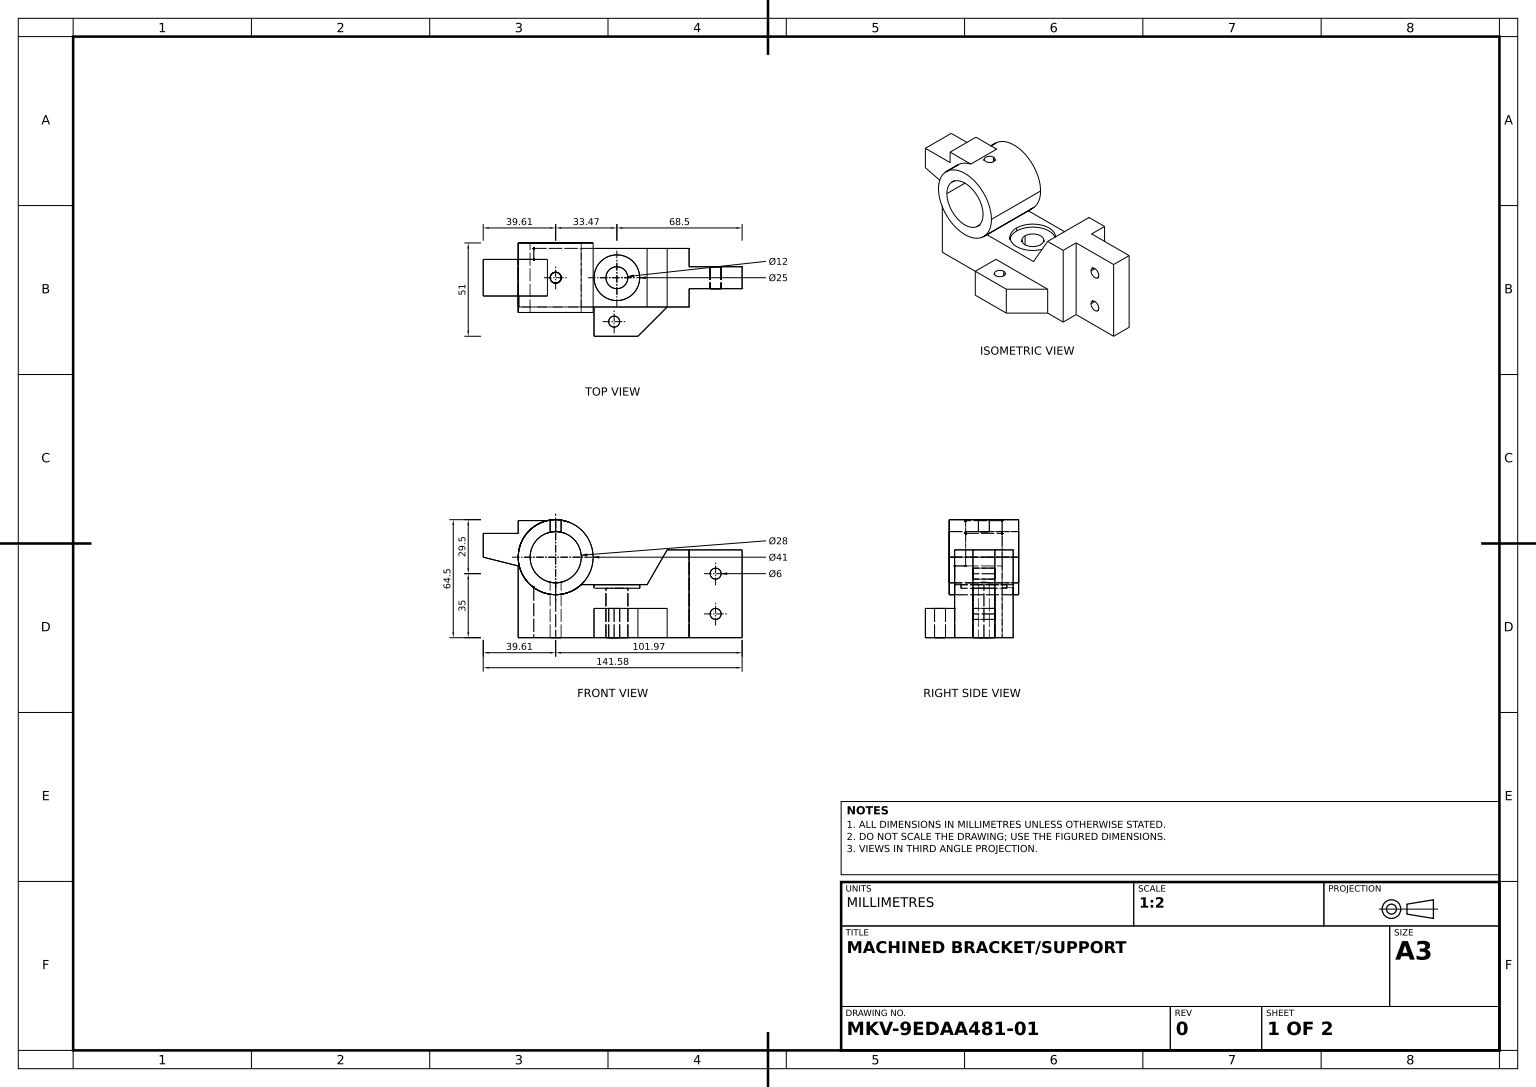
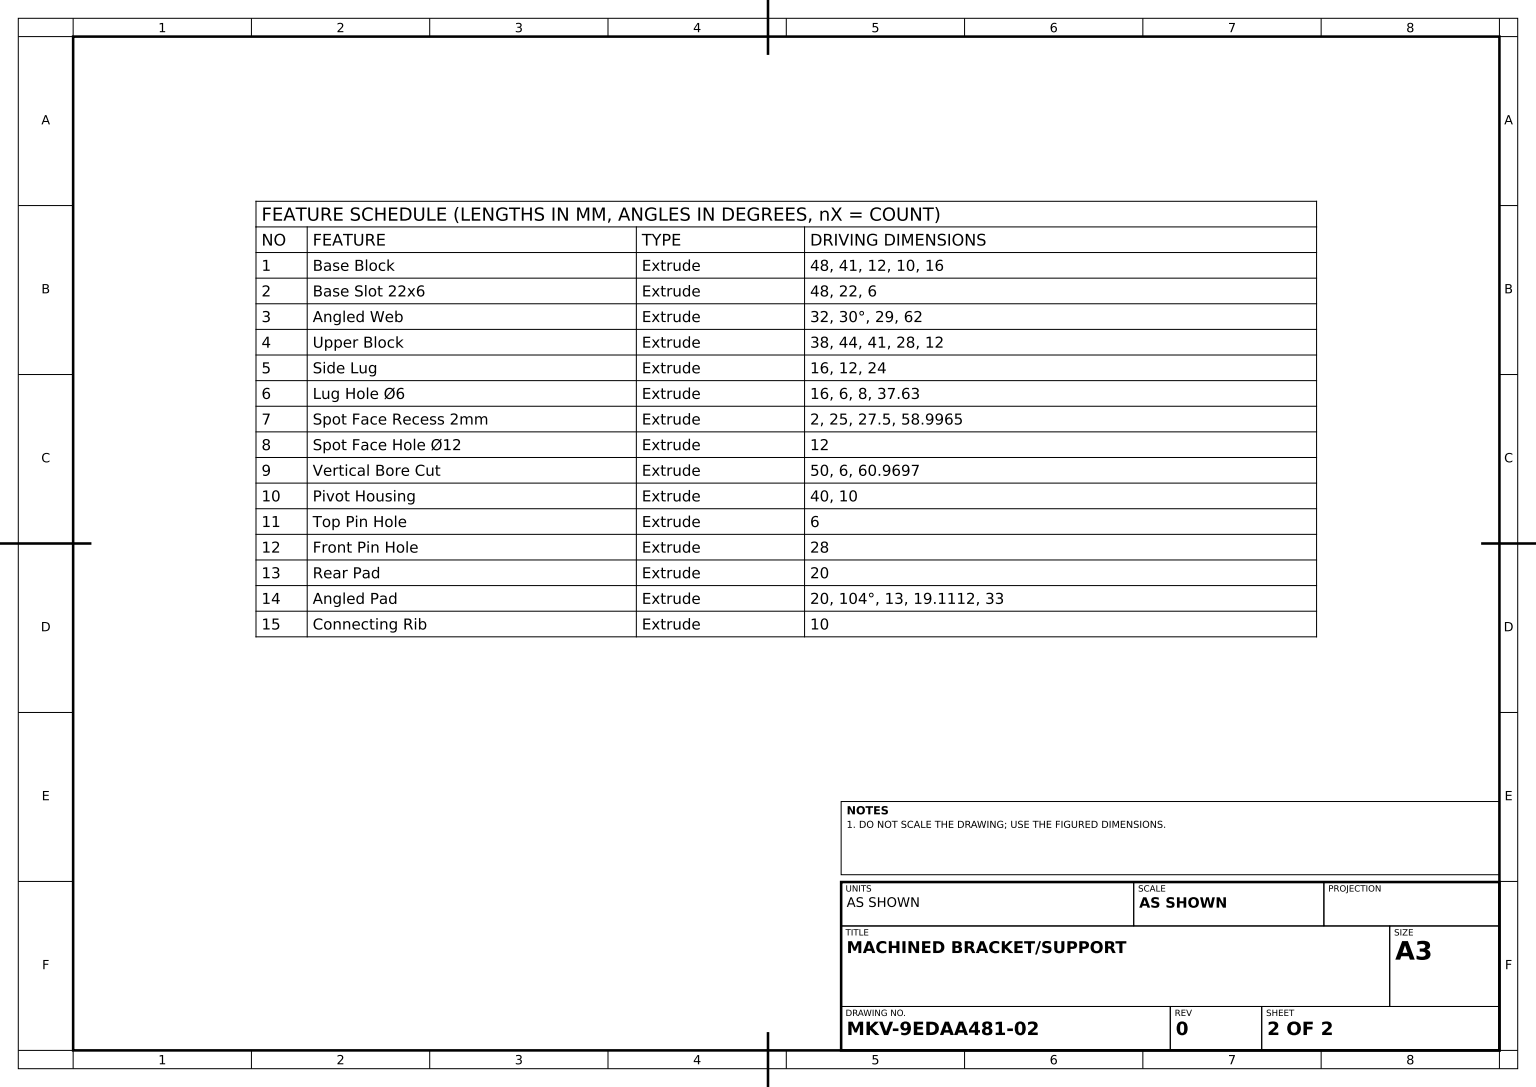
SolidWorks part; units mm, degrees
material "Plain Carbon Steel"
ref_plane "Front Plane" through (0, 0, 0) normal (0, 0, 1) x (1, 0, 0)
ref_plane "Top Plane" through (0, 0, 0) normal (0, 1, 0) x (1, 0, 0)
ref_plane "Right Plane" through (0, 0, 0) normal (1, 0, 0) x (0, 0, -1)
sketch "Base Block Sketch" plane through (0, 0, 0) normal (0, 1, 0) x (1, 0, 0)
  line L0 (0, -16) -> (0, 16)
  line L1 (0, 16) -> (12, 16)
  line L2 (12, 6) -> (41, 6)
  line L3 (0, 0) -> (38.6763, 0) construction
  line L4 (0, -16) -> (12, -16)
  line L5 (12, -16) -> (12, -6)
  line L6 (12, -6) -> (41, -6)
  line L7 (12, 16) -> (12, 6)
  line L8 (41, 6) -> (41, -6)
  dimension "D1" = 41
  dimension "D2" = 12
  dimension "D3" = 10
  dimension "D4" = 16
extrude "Base Block" add sketch "Base Block Sketch" against normal mid plane 48
sketch "Base Slot Sketch" plane through (0, 0, 6) normal (0, 0, 1) x (1, 0, 0)
  line L0 (0, 0) -> (41, 0) construction
  line L1 (41, -24) -> (41, 24) construction
  line L2 (26.5, 24) -> (26.5, 11) construction
  line L3 (12, 24) -> (41, 24) construction
  circle A0 centre (26.5, 11) radius 3
  circle A1 centre (26.5, -11) radius 3
  dimension "D1" = 22
  dimension "D2" = 6
extrude "Base Slot 22x6" cut sketch "Base Slot Sketch" against normal blind 48
sketch "Angled Web Sketch" plane through (0, 0, 0) normal (0, 0, 1) x (1, 0, 0)
  line L0 (0, -24) -> (0, 5) construction
  line L1 (0, -24) -> (0, 24) construction
  line L2 (0, 5) -> (-70.4973, 5) construction
  line L3 (0, -24) -> (0, 24)
  line L4 (0, 24) -> (-10.9697, 5)
  line L5 (-10.9697, 5) -> (-72.9697, 5)
  line L6 (-72.9697, 5) -> (-72.9697, -24)
  line L7 (-72.9697, -24) -> (0, -24)
  dimension "D1" = 30
  dimension "D2" = 29
  dimension "D3" = 62
extrude "Angled Web" add sketch "Angled Web Sketch" along normal mid plane 32
sketch "Upper Block Sketch" plane through (0, 0, 0) normal (0, 0, 1) x (1, 0, 0)
  line L0 (-72.9697, -24) -> (-60.9697, -24) construction
  line L1 (-72.9697, -24) -> (12, -24) construction
  line L2 (-60.9697, -24) -> (-60.9697, 20) construction
  circle A0 centre (-60.9697, 20) radius 20.5
  circle A1 centre (-60.9697, 20) radius 14
  dimension "D1" = 44
  dimension "D2" = 41
  dimension "D3" = 28
  dimension "D4" = 12
extrude "Upper Block" add sketch "Upper Block Sketch" along normal mid plane 38
sketch "Side Lug Sketch" plane through (0, -24, 0) normal (0, -1, 0) x (1, 0, 0)
  line L0 (12, 16) -> (0, 16)
  line L1 (-72.9697, 16) -> (12, 16) construction
  line L2 (0, 16) -> (-16, 32)
  line L3 (-16, 32) -> (-16, 16)
  line L4 (-16, 32) -> (-40, 32)
  line L5 (-40, 32) -> (-40, 16)
  line L6 (-40, 16) -> (0, 16)
  line M9 (12, 16) -> (-72.9697, 16)
  dimension "D1" = 16
  dimension "D2" = 16
  dimension "D3" = 12
  dimension "D4" = 24
extrude "Side Lug" add sketch "Side Lug Sketch" against normal blind 16 contours L4 L5 L3 M9 | L2 L3 M9
sketch "Lug Hole Sketch" plane through (0, -8, 0) normal (0, 1, 0) x (1, 0, 0)
  line L0 (-10.9697, -16) -> (-46.9965, -16) construction
  circle A0 centre (-28.9831, -24) radius 3
  dimension "D1" = 6
  dimension "D2" = 8
  dimension "D3" = 37.63
extrude "Lug Hole Ø6" cut sketch "Lug Hole Sketch" against normal blind 16
sketch "Spot Face Recess Sketch" plane through (0, 5, 0) normal (0, 1, 0) x (1, 0, 0)
  line L0 (12, 0) -> (41, 0)
  line L1 (-46.9965, -16) -> (-46.9965, 16) construction
  line L2 (41, -6) -> (41, 6) construction
  line L3 (26.5, 0) -> (-27.5, 0) construction
  circle A0 centre (-27.5, 0) radius 12.5
  point P5 (26.5, 0)
  dimension "D1" = 25
  dimension "D2" = 27.5
  dimension "D3" = 58.9965
extrude "Spot Face Recess 2mm" cut sketch "Spot Face Recess Sketch" against normal blind 2
sketch "Spot Face Hole Sketch" plane through (0, 3, 0) normal (0, 1, 0) x (1, 0, 0)
  circle A0 centre (-27.5, 0) radius 6
  dimension "D1" = 12
extrude "Spot Face Hole Ø12" cut sketch "Spot Face Hole Sketch" against normal through all
sketch "Vertical Bore Sketch" plane through (0, 0, 0) normal (0, 1, 0) x (1, 0, 0)
  circle A0 centre (-60.9697, 0) radius 3
  dimension "D1" = 6
  dimension "D2" = 60.9697
extrude "Vertical Bore Cut" cut sketch "Vertical Bore Sketch" along normal blind 50
sketch "Pivot Housing Sketch" plane through (0, 0, 0) normal (0, 1, 0) x (1, 0, 0)
  line L0 (-60.9697, 0) -> (-60.9697, 10)
  line L1 (-60.9697, 10) -> (-81.4697, 10)
  line L2 (-81.4697, 19) -> (-81.4697, -19) construction
  line L3 (-81.4697, 10) -> (-81.4697, -10)
  line L4 (-81.4697, -10) -> (-60.9697, -10)
  line L5 (-60.9697, -10) -> (-60.9697, 0)
  dimension "D1" = 10
extrude "Pivot Housing" add sketch "Pivot Housing Sketch" along normal blind 40
sketch "Top Pin Hole Sketch" plane through (0, 0, 0) normal (0, 1, 0) x (1, 0, 0)
  line L0 (-60.9697, -3) -> (-60.9697, 3) construction
  circle A0 centre (-60.9697, 0) radius 3
  dimension "D1" = 6
extrude "Top Pin Hole" cut sketch "Top Pin Hole Sketch" against normal through all both and the other way through all
sketch "Front Pin Hole Sketch" plane through (0, 0, 0) normal (0, 0, 1) x (1, 0, 0)
  line L0 (-60.9697, 34) -> (-60.9697, 6) construction
  circle A0 centre (-60.9697, 20) radius 14
  dimension "D1" = 28
extrude "Front Pin Hole" cut sketch "Front Pin Hole Sketch" against normal through all both and the other way through all
sketch "Rear Pad Sketch" plane through (0, 0, 10) normal (0, 0, 1) x (1, 0, 0)
  line L0 (-81.4697, 0) -> (-72.9697, 0)
  line L1 (-72.9697, 0) -> (-72.9697, -24)
  line L2 (-72.9697, -24) -> (-81.4697, -24)
  line L3 (-81.4697, -24) -> (-81.4697, 0)
extrude "Rear Pad" add sketch "Rear Pad Sketch" against normal blind 20
sketch "Angled Pad Sketch" plane through (0, 0, 0) normal (0, 0, 1) x (1, 0, 0)
  line L1 (-100.5809, 20) -> (-100.5809, 33)
  line L2 (-100.5809, 33) -> (-81.4697, 33)
  line L3 (-81.4697, 40) -> (-81.4697, 20) construction
  line L4 (-81.4697, 33) -> (-81.4697, 15.235)
  line L5 (-81.4697, 20) -> (-81.4697, -24) construction
  line L6 (-81.4697, 15.235) -> (-100.5809, 20)
  dimension "D1" = 104
  dimension "D2" = 13
  dimension "D3" = 19.1112
  dimension "D4" = 33
extrude "Angled Pad" add sketch "Angled Pad Sketch" along normal mid plane 20
sketch "Connecting Rib Sketch" plane through (0, 0, 16) normal (0, 0, 1) x (1, 0, 0)
  line L0 (-72.9697, -24) -> (-81.4697, -24)
  line L1 (-81.4697, -24) -> (-72.9697, -24) construction
  line L2 (-81.4697, 15.235) -> (-81.4697, -24) construction
  line L3 (-81.4697, -24) -> (-81.4697, 15.235)
  line L4 (-100.5809, 20) -> (-81.4697, 15.235) construction
  line L5 (-81.4697, 15.235) -> (-80.9082, 15.235)
  line L6 (-72.9697, -24) -> (-72.9697, 3.3792)
  arc A1 (-80.9082, 15.235) -> (-72.9697, 3.3792) centre (-60.9697, 20) ccw
extrude "Connecting Rib" add sketch "Connecting Rib Sketch" against normal blind 10
